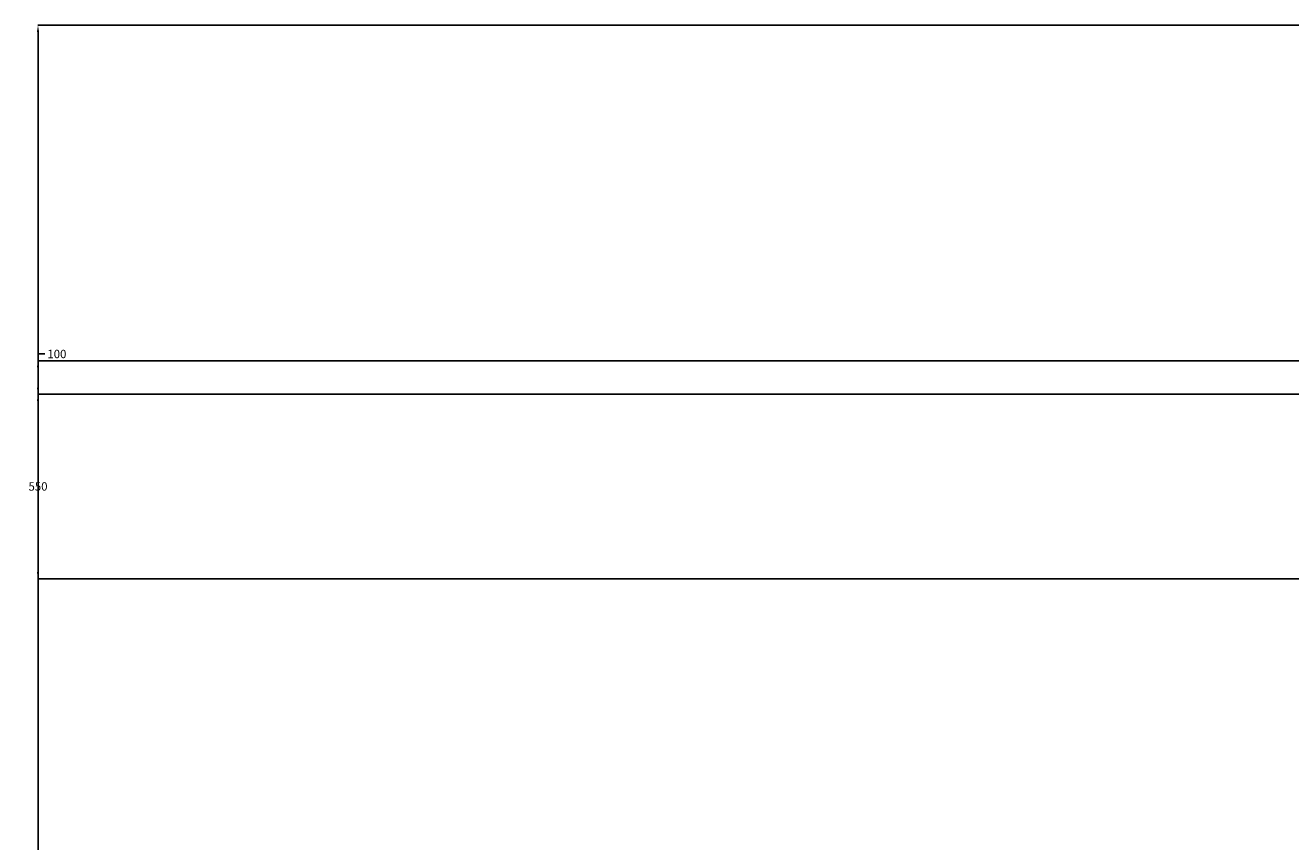
# Model space of a CAD drawing. Units: millimetres. Extents: x -692 to 9639, y -141 to 10345.
# Tile 12 of 19: x -687 to 3088, y 7415 to 9849. Entities that reach past the tile are written whole.
import ezdxf

# ---------------------------------------------------------------- set-up
doc = ezdxf.new("R2010")
doc.units = ezdxf.units.MM
doc.header["$MEASUREMENT"] = 0
doc.layers.add('A-ANNO-DIMS', color=2, linetype='Continuous', lineweight=18)
doc.styles.get("Standard").update_dxf_attribs({"font": 'arial.ttf'})
doc.dimstyles.get("Standard").update_dxf_attribs({"dimtxt": 25, "dimasz": 20, "dimexe": 0.18, "dimexo": 10, "dimgap": 10, "dimtad": 0, "dimtih": 1, "dimtoh": 1, "dimdec": 0, "dimzin": 0, "dimdsep": 46, "dimtxsty": 'Standard', "dimcen": 10, "dimadec": 0, "dimazin": 0, "dimtfac": 1, "dimtdec": 0, "dimtofl": 0, "dimtmove": 0, "dimatfit": 3, "dimfxl": 1, "dimtolj": 1, "dimtzin": 0, "dimarcsym": 0})

# ---------------------------------------------------------------- blocks, each defined once
blk = doc.blocks.new('*D7')
at = {"layer": 'A-ANNO-DIMS', "color": 0, "lineweight": -2, "transparency": 16777216}
for p, q in [((8481.5, 9848.8), (-649.1, 9848.8)), ((-648.9, 9828.8), (-648.9, 5124.9)), ((-648.9, 375.6), (-648.9, 5079.4)), ((2463.7, 355.6), (-649.1, 355.6))]:
    blk.add_line(p, q, dxfattribs=at)
at = {"layer": 'A-ANNO-DIMS', "color": 0, "lineweight": -3, "transparency": 16777216}
for points in [[(-652.2, 9828.8), (-645.6, 9828.8), (-648.9, 9848.8)], [(-652.2, 375.6), (-645.6, 375.6), (-648.9, 355.6)]]:
    blk.add_solid(points, dxfattribs=at)
at = {"layer": 'Defpoints', "color": 0, "lineweight": -3, "transparency": 16777216}
for p in [(-648.9, 9848.8), (8491.5, 9848.8), (2473.7, 355.6)]:
    blk.add_point(p, dxfattribs=at)
at = {"layer": 'A-ANNO-DIMS', "color": 0, "transparency": 16777216, "insert": (-648.9, 5102.2), "char_height": 25, "attachment_point": 5}
blk.add_mtext('\\A1;9493', dxfattribs=at)
blk = doc.blocks.new('*D69')
at = {"layer": 'A-ANNO-DIMS', "color": 0, "lineweight": -2, "transparency": 16777216}
for p, q in [((3781.5, 8748.8), (-649.1, 8748.8)), ((-648.9, 8728.8), (-648.9, 8496.5)), ((-648.9, 8218.8), (-648.9, 8451)), ((3931.5, 8198.8), (-649.1, 8198.8))]:
    blk.add_line(p, q, dxfattribs=at)
at = {"layer": 'A-ANNO-DIMS', "color": 0, "lineweight": -3, "transparency": 16777216}
for points in [[(-652.2, 8728.8), (-645.6, 8728.8), (-648.9, 8748.8)], [(-652.2, 8218.8), (-645.6, 8218.8), (-648.9, 8198.8)]]:
    blk.add_solid(points, dxfattribs=at)
at = {"layer": 'Defpoints', "color": 0, "lineweight": -3, "transparency": 16777216}
for p in [(-648.9, 8748.8), (3791.5, 8748.8), (3941.5, 8198.8)]:
    blk.add_point(p, dxfattribs=at)
at = {"layer": 'A-ANNO-DIMS', "color": 0, "transparency": 16777216, "insert": (-648.9, 8473.8), "char_height": 25, "attachment_point": 5}
blk.add_mtext('\\A1;550', dxfattribs=at)
blk = doc.blocks.new('*D70')
at = {"layer": 'A-ANNO-DIMS', "color": 0, "lineweight": -2, "transparency": 16777216}
for p, q in [((3781.5, 8848.8), (-649.1, 8848.8)), ((-648.9, 8848.8), (-648.9, 8868.8)), ((-648.9, 8868.8), (-628.9, 8868.8)), ((-648.9, 8768.8), (-648.9, 8828.8)), ((3781.5, 8748.8), (-649.1, 8748.8))]:
    blk.add_line(p, q, dxfattribs=at)
at = {"layer": 'A-ANNO-DIMS', "color": 0, "lineweight": -3, "transparency": 16777216}
for points in [[(-652.2, 8828.8), (-645.6, 8828.8), (-648.9, 8848.8)], [(-652.2, 8768.8), (-645.6, 8768.8), (-648.9, 8748.8)]]:
    blk.add_solid(points, dxfattribs=at)
at = {"layer": 'Defpoints', "color": 0, "lineweight": -3, "transparency": 16777216}
for p in [(-648.9, 8848.8), (3791.5, 8848.8), (3791.5, 8748.8)]:
    blk.add_point(p, dxfattribs=at)
at = {"layer": 'A-ANNO-DIMS', "color": 0, "transparency": 16777216, "insert": (-592.5, 8868.8), "char_height": 25, "attachment_point": 5}
blk.add_mtext('\\A1;100', dxfattribs=at)

msp = doc.modelspace()

# ---------------------------------------------------------------- dimensions: what is measured, and where the dimension line sits
at = {"layer": 'A-ANNO-DIMS'}
for base, p1, p2, picture, middle in [((-648.912, 9848.772), (2473.746, 355.575), (8491.547, 9848.772), '*D7', (-648.912, 5102.173)), ((-648.912, 8848.772), (3791.547, 8748.772), (3791.547, 8848.772), '*D70', (-592.514, 8868.772)), ((-648.912, 8748.772), (3941.547, 8198.772), (3791.547, 8748.772), '*D69', (-648.912, 8473.772))]:
    dim = msp.add_linear_dim(base=base, p1=p1, p2=p2, angle=90, dimstyle='Standard', override={"dimdec": 0, "dimlfac": 1, "dimrnd": 0, "dimzin": 0, "dimdsep": 46, "dimlunit": 2}, dxfattribs=at)
    dim.commit()
    dim.dimension.update_dxf_attribs({"geometry": picture, "text_midpoint": middle})

doc.saveas('drawing.dxf')
